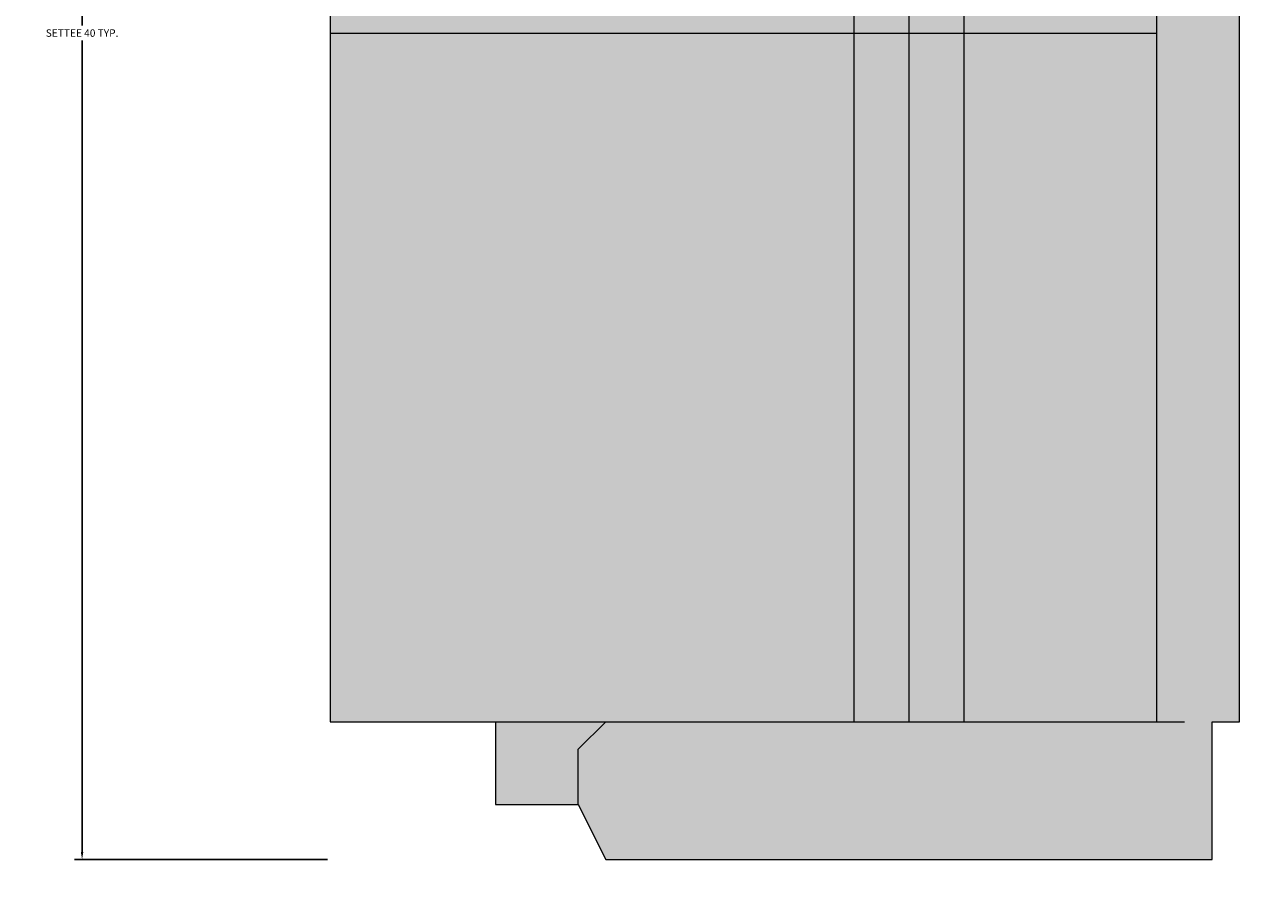
# Model space of a CAD drawing. Units: millimetres. Extents: x 27017497 to 27018854, y 7058029 to 7059154.
# Tile 55 of 91: x 27017980 to 27018010, y 7058327 to 7058348. Entities that reach past the tile are written whole.
import ezdxf

# ---------------------------------------------------------------- set-up
doc = ezdxf.new("R2010")
doc.units = ezdxf.units.MM
doc.layers.add('A-ANNO-DIMS', color=2, linetype='Continuous', lineweight=18)
doc.layers.add('A-FURN', color=8, linetype='Continuous', lineweight=18)
doc.layers.add('A-FURN-PATT', color=177, linetype='Continuous', lineweight=13, true_color=0x293189)
doc.styles.get("Standard").update_dxf_attribs({"font": 'arial.ttf'})
doc.dimstyles.get("Standard").update_dxf_attribs({"dimtxt": 0.18, "dimasz": 0.18, "dimexe": 0.18, "dimexo": 0.0625, "dimgap": 0.09, "dimtad": 0, "dimtih": 1, "dimtoh": 1, "dimdec": 4, "dimzin": 0, "dimdsep": 46, "dimtxsty": 'Standard', "dimcen": 0.09, "dimadec": 0, "dimazin": 0, "dimtfac": 1, "dimtdec": 4, "dimtofl": 0, "dimtmove": 0, "dimatfit": 3, "dimfxl": 1, "dimtolj": 1, "dimtzin": 0, "dimarcsym": 0})

# ---------------------------------------------------------------- blocks, each defined once
blk = doc.blocks.new('SETTEE-TWO-SEAT')
for p, q in [((6.669, 40.014), (6.002, 38.68)), ((21.34, 40.014), (6.669, 40.014)), ((21.34, 36.679), (21.34, 40.014)), ((6.002, 38.68), (4.001, 38.68)), ((4.001, 38.68), (4.001, 36.679)), ((6.002, 38.68), (6.002, 37.346)), ((6.002, 37.346), (6.669, 36.679)), ((0, 36.679), (0, 3.334)), ((4.001, 36.679), (0, 36.679)), ((4.001, 36.679), (6.669, 36.679)), ((6.669, 36.679), (20.673, 36.679)), ((12.671, 36.679), (12.671, 3.334)), ((14.004, 36.679), (14.004, 3.334)), ((15.338, 36.679), (15.338, 3.334)), ((20.006, 3.334), (20.006, 36.679)), ((22.007, 36.679), (21.34, 36.679)), ((22.007, 3.334), (22.007, 36.679)), ((0, 20.007), (20.006, 20.007)), ((0, 3.334), (4.001, 3.334)), ((4.001, 3.334), (6.669, 3.334)), ((4.001, 3.334), (4.001, 1.334)), ((6.002, 2.668), (6.669, 3.334)), ((6.669, 3.334), (20.673, 3.334)), ((21.34, 0), (21.34, 3.334)), ((21.34, 3.334), (22.007, 3.334)), ((6.002, 1.334), (6.002, 2.668)), ((4.001, 1.334), (6.002, 1.334)), ((6.002, 1.334), (6.669, 0)), ((6.669, 0), (21.34, 0))]:
    blk.add_line(p, q)
blk = doc.blocks.new('*D27')
at = {"layer": 'A-ANNO-DIMS', "color": 0, "lineweight": -2, "transparency": 16777216}
for p, q in [((27017987.706, 7058367.587), (27017981.587, 7058367.587)), ((27017981.767, 7058367.407), (27017981.767, 7058347.763)), ((27017981.767, 7058327.753), (27017981.767, 7058347.397)), ((27017987.706, 7058327.573), (27017981.587, 7058327.573))]:
    blk.add_line(p, q, dxfattribs=at)
at = {"layer": 'A-ANNO-DIMS', "color": 0, "transparency": 16777216}
for points in [[(27017981.737, 7058367.407), (27017981.797, 7058367.407), (27017981.767, 7058367.587)], [(27017981.737, 7058327.753), (27017981.797, 7058327.753), (27017981.767, 7058327.573)]]:
    blk.add_solid(points, dxfattribs=at)
at = {"layer": 'Defpoints', "color": 0, "transparency": 16777216}
for p in [(27017981.767, 7058367.587), (27017987.769, 7058367.587), (27017987.769, 7058327.573)]:
    blk.add_point(p, dxfattribs=at)
at = {"layer": 'A-ANNO-DIMS', "color": 0, "transparency": 16777216, "insert": (27017981.767, 7058347.58), "char_height": 0.18, "attachment_point": 5}
blk.add_mtext('\\A1;SETTEE 40 TYP.', dxfattribs=at)
blk = doc.blocks.new('*D48')
at = {"layer": 'A-ANNO-DIMS', "color": 0, "lineweight": -2, "transparency": 16777216}
for p, q in [((27018463.498, 7058622.912), (27017497.536, 7058622.912)), ((27017497.716, 7058622.732), (27017497.716, 7058357.753)), ((27017497.716, 7058092.41), (27017497.716, 7058357.389)), ((27018555.129, 7058092.23), (27017497.536, 7058092.23))]:
    blk.add_line(p, q, dxfattribs=at)
at = {"layer": 'A-ANNO-DIMS', "color": 0, "transparency": 16777216}
for points in [[(27017497.686, 7058622.732), (27017497.746, 7058622.732), (27017497.716, 7058622.912)], [(27017497.686, 7058092.41), (27017497.746, 7058092.41), (27017497.716, 7058092.23)]]:
    blk.add_solid(points, dxfattribs=at)
at = {"layer": 'Defpoints', "color": 0, "transparency": 16777216}
for p in [(27018463.561, 7058622.912), (27017497.716, 7058092.23), (27018555.192, 7058092.23)]:
    blk.add_point(p, dxfattribs=at)
at = {"layer": 'A-ANNO-DIMS', "color": 0, "transparency": 16777216, "insert": (27017497.716, 7058357.571), "char_height": 0.18, "attachment_point": 5}
blk.add_mtext('\\A1;530.7', dxfattribs=at)

msp = doc.modelspace()

# ---------------------------------------------------------------- hatches: boundary and pattern name
at = {"layer": 'A-FURN-PATT'}
h = msp.add_hatch(color=256, dxfattribs=at)
h.dxf.hatch_style = 1
h.paths.add_polyline_path([(27017921.559, 7058320.14), (27017906.276, 7058320.14), (27017906.276, 7058304.857), (27017921.559, 7058304.857)])
h.paths.add_polyline_path([(27017921.003, 7058319.584), (27017921.003, 7058305.412), (27017906.831, 7058305.412), (27017906.831, 7058319.584)], flags=16)
h.paths.add_polyline_path([(27017918.811, 7058312.427, -1), (27017909.19, 7058312.427, -1)], flags=0)
h.paths.add_polyline_path([(27017919.33, 7058326.783), (27017919.33, 7058328.117), (27017918.663, 7058328.784), (27017905.325, 7058328.784), (27017905.325, 7058362.129), (27017918.663, 7058362.129), (27017919.33, 7058362.796), (27017919.33, 7058364.13), (27017918.663, 7058365.463), (27017903.991, 7058365.463), (27017903.991, 7058362.129), (27017903.325, 7058362.129), (27017903.325, 7058328.784), (27017903.991, 7058328.784), (27017903.991, 7058325.45), (27017918.663, 7058325.45)])
h.paths.add_polyline_path([(27017925.332, 7058345.456), (27017912.661, 7058345.456), (27017912.661, 7058328.784), (27017918.663, 7058328.784), (27017921.331, 7058328.784), (27017925.332, 7058328.784)])
h.paths.add_polyline_path([(27017925.332, 7058362.129), (27017921.331, 7058362.129), (27017918.663, 7058362.129), (27017912.661, 7058362.129), (27017912.661, 7058345.456), (27017925.332, 7058345.456)])
h.paths.add_polyline_path([(27017909.993, 7058362.129), (27017905.325, 7058362.129), (27017905.325, 7058345.456), (27017909.993, 7058345.456)], flags=17)
h.paths.add_polyline_path([(27017909.993, 7058345.456), (27017905.325, 7058345.456), (27017905.325, 7058328.784), (27017909.993, 7058328.784)], flags=17)
h.paths.add_polyline_path([(27017911.327, 7058345.456), (27017909.993, 7058345.456), (27017909.993, 7058328.784), (27017911.327, 7058328.784)], flags=17)
h.paths.add_polyline_path([(27017912.661, 7058345.456), (27017911.327, 7058345.456), (27017911.327, 7058328.784), (27017912.661, 7058328.784)], flags=17)
h.paths.add_polyline_path([(27017912.661, 7058362.129), (27017911.327, 7058362.129), (27017911.327, 7058345.456), (27017912.661, 7058345.456)], flags=17)
h.paths.add_polyline_path([(27017911.327, 7058362.129), (27017909.993, 7058362.129), (27017909.993, 7058345.456), (27017911.327, 7058345.456)], flags=17)
h.paths.add_polyline_path([(27017973.504, 7058350.536), (27017940.159, 7058350.536), (27017940.159, 7058333.863), (27017973.504, 7058333.863)])
h.paths.add_polyline_path([(27017972.67, 7058349.702), (27017972.67, 7058334.697), (27017940.993, 7058334.697), (27017940.993, 7058349.702)], flags=16)
h.paths.add_polyline_path([(27018000.44, 7058364.252), (27017994.438, 7058364.252), (27017991.77, 7058364.252), (27017987.769, 7058364.252), (27017987.769, 7058347.58), (27018000.44, 7058347.58)])
h.paths.add_polyline_path([(27018000.44, 7058347.58), (27017987.769, 7058347.58), (27017987.769, 7058330.907), (27017991.77, 7058330.907), (27017994.438, 7058330.907), (27018000.44, 7058330.907)])
h.paths.add_polyline_path([(27018009.109, 7058330.907), (27018009.776, 7058330.907), (27018009.776, 7058364.252), (27018009.109, 7058364.252), (27018009.109, 7058367.587), (27017994.438, 7058367.587), (27017993.771, 7058366.253), (27017993.771, 7058364.919), (27017994.438, 7058364.252), (27018007.775, 7058364.252), (27018007.775, 7058330.907), (27017994.438, 7058330.907), (27017993.771, 7058330.241), (27017993.771, 7058328.907), (27017994.438, 7058327.573), (27018009.109, 7058327.573)])
h.paths.add_polyline_path([(27017994.438, 7058330.907), (27017991.77, 7058330.907), (27017991.77, 7058328.907), (27017993.771, 7058328.907), (27017993.771, 7058330.241)])
h.paths.add_polyline_path([(27017993.771, 7058366.253), (27017991.77, 7058366.253), (27017991.77, 7058364.252), (27017994.438, 7058364.252), (27017993.771, 7058364.919)])
h.paths.add_polyline_path([(27018007.775, 7058364.252), (27018003.107, 7058364.252), (27018003.107, 7058347.58), (27018007.775, 7058347.58)], flags=17)
h.paths.add_polyline_path([(27018007.775, 7058347.58), (27018003.107, 7058347.58), (27018003.107, 7058330.907), (27018007.775, 7058330.907)], flags=17)
h.paths.add_polyline_path([(27018003.107, 7058364.252), (27018001.773, 7058364.252), (27018001.773, 7058347.58), (27018003.107, 7058347.58)], flags=17)
h.paths.add_polyline_path([(27018003.107, 7058347.58), (27018001.773, 7058347.58), (27018001.773, 7058330.907), (27018003.107, 7058330.907)], flags=17)
h.paths.add_polyline_path([(27018001.773, 7058347.58), (27018000.44, 7058347.58), (27018000.44, 7058330.907), (27018001.773, 7058330.907)], flags=17)
h.paths.add_polyline_path([(27018001.773, 7058364.252), (27018000.44, 7058364.252), (27018000.44, 7058347.58), (27018001.773, 7058347.58)], flags=17)

# ---------------------------------------------------------------- block references
at = {"layer": 'A-FURN'}
msp.add_blockref('SETTEE-TWO-SEAT', (27017987.769, 7058327.573), dxfattribs=at)

# ---------------------------------------------------------------- dimensions: what is measured, and where the dimension line sits
at = {"layer": 'A-ANNO-DIMS'}
dim = msp.add_linear_dim(base=(27017497.716, 7058092.23), p1=(27018463.561, 7058622.912), p2=(27018555.192, 7058092.23), angle=90, dimstyle='Standard', override={"dimdec": 1, "dimlfac": 1, "dimrnd": 0, "dimzin": 0, "dimdsep": 46, "dimlunit": 2}, dxfattribs=at)
dim.commit()
dim.dimension.update_dxf_attribs({"geometry": '*D48', "text_midpoint": (27017497.716, 7058357.571)})
dim = msp.add_linear_dim(base=(27017981.767, 7058367.587), p1=(27017987.769, 7058327.573), p2=(27017987.769, 7058367.587), angle=90, text='SETTEE <> TYP.', dimstyle='Standard', override={"dimdec": 0, "dimlfac": 1, "dimrnd": 0, "dimzin": 0, "dimdsep": 46, "dimlunit": 2}, dxfattribs=at)
dim.commit()
dim.dimension.update_dxf_attribs({"geometry": '*D27', "text_midpoint": (27017981.767, 7058347.58)})

doc.saveas('drawing.dxf')
